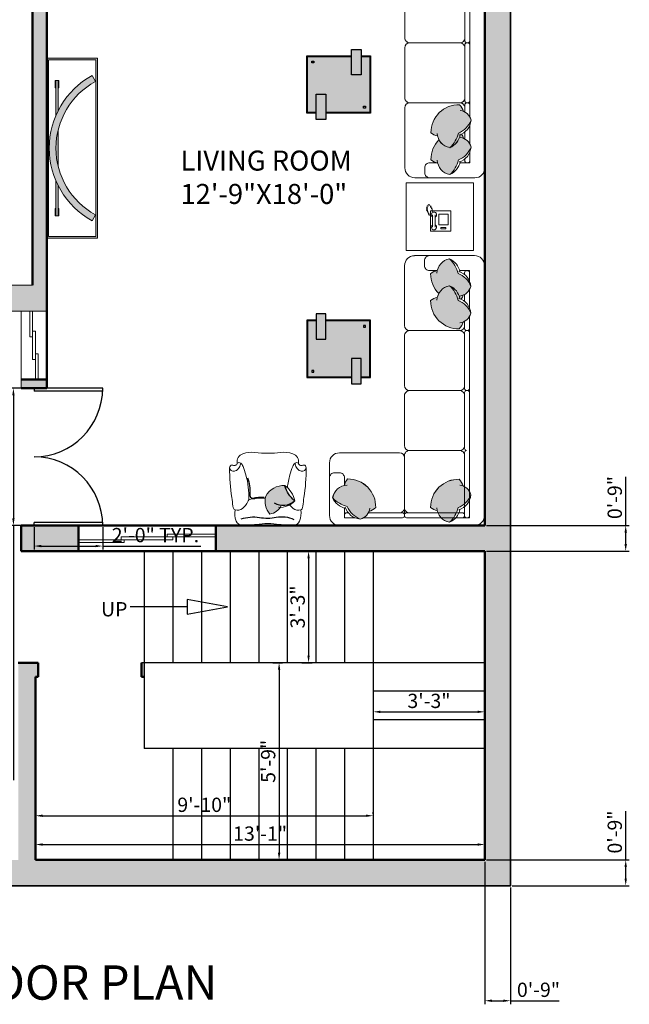
# Model space of a CAD drawing. Units: inches. Extents: x 1734 to 4011, y 1071 to 1891.
# Tile 2 of 27: x 1947 to 2160, y 1083 to 1427. Entities that reach past the tile are written whole.
import ezdxf

# ---------------------------------------------------------------- set-up
doc = ezdxf.new("R2010")
doc.units = ezdxf.units.IN
for name, color, linetype, lineweight in [('A-ANNO-DIMS', 2, 'Continuous', 18), ('A-ANNO-TEXT', 7, 'Continuous', 25), ('A-AREA-IDEN', 3, 'Continuous', 18), ('A-DOOR', 3, 'Continuous', 25), ('A-FLOR-STRS', 2, 'Continuous', 25), ('A-FURN', 8, 'Continuous', 18), ('A-FURN-PATT', 252, 'Continuous', 13), ('A-GLAZ', 4, 'Continuous', 18), ('A-WALL', 7, 'Continuous', 50), ('A-WALL-PATT', 8, 'Continuous', 13), ('aparador', 36, 'Continuous', 9), ('C-PROP', 1, 'Continuous', 35), ('moveis', 254, 'Continuous', 5)]:
    doc.layers.add(name, color=color, linetype=linetype, lineweight=lineweight)
doc.layers.add('IFF-FURN-DETAIL', color=250, linetype='Continuous')
doc.layers.add('MOBIL', color=7, linetype='Continuous')
doc.styles.get("Standard").update_dxf_attribs({"font": 'arial.ttf'})
doc.dimstyles.new('ISO-25', dxfattribs={"dimtxt": 5, "dimasz": 2.5, "dimexe": 1.25, "dimexo": 0.625, "dimtad": 1, "dimdec": 1, "dimlunit": 3, "dimtxsty": 'Standard', "dimcen": 2.5, "dimclrt": 1, "dimadec": 0, "dimazin": 0, "dimtfac": 1, "dimtdec": 1, "dimtmove": 0, "dimatfit": 3, "dimfxl": 1, "dimarcsym": 0})

# ---------------------------------------------------------------- blocks, each defined once
blk = doc.blocks.new('*D8')
at = {"layer": 'A-ANNO-DIMS', "color": 0, "lineweight": -2, "transparency": 16777216}
for p, q in [((2045.72, 1241.06), (2049.34, 1241.06)), ((2048.09, 1238.56), (2048.09, 1204.56)), ((2045.72, 1202.06), (2049.34, 1202.06))]:
    blk.add_line(p, q, dxfattribs=at)
at = {"layer": 'A-ANNO-DIMS', "color": 0, "transparency": 16777216}
for points in [[(2047.67, 1238.56), (2048.5, 1238.56), (2048.09, 1241.06)], [(2047.67, 1204.56), (2048.5, 1204.56), (2048.09, 1202.06)]]:
    blk.add_solid(points, dxfattribs=at)
at = {"layer": 'Defpoints', "color": 0, "transparency": 16777216}
for p in [(2045.09, 1241.06), (2045.09, 1202.06), (2048.09, 1202.06)]:
    blk.add_point(p, dxfattribs=at)
at = {"layer": 'A-ANNO-DIMS', "color": 0, "transparency": 16777216, "insert": (2044.91, 1221.56), "char_height": 5, "attachment_point": 5, "rotation": 90}
blk.add_mtext('3\'-3"', dxfattribs=at)
blk = doc.blocks.new('*D9')
at = {"layer": 'A-ANNO-DIMS', "color": 0, "lineweight": -2, "transparency": 16777216}
for p, q in [((2035.64, 1202.06), (2039.03, 1202.06)), ((2037.78, 1199.56), (2037.78, 1135.56)), ((2035.64, 1133.06), (2039.03, 1133.06))]:
    blk.add_line(p, q, dxfattribs=at)
at = {"layer": 'A-ANNO-DIMS', "color": 0, "transparency": 16777216}
for points in [[(2037.37, 1199.56), (2038.2, 1199.56), (2037.78, 1202.06)], [(2037.37, 1135.56), (2038.2, 1135.56), (2037.78, 1133.06)]]:
    blk.add_solid(points, dxfattribs=at)
at = {"layer": 'Defpoints', "color": 0, "transparency": 16777216}
for p in [(2035.02, 1202.06), (2035.02, 1133.06), (2037.78, 1133.06)]:
    blk.add_point(p, dxfattribs=at)
at = {"layer": 'A-ANNO-DIMS', "color": 0, "transparency": 16777216, "insert": (2034.61, 1167.56), "char_height": 5, "attachment_point": 5, "rotation": 90}
blk.add_mtext('5\'-9"', dxfattribs=at)
blk = doc.blocks.new('*D10')
at = {"layer": 'A-ANNO-DIMS', "color": 0, "lineweight": -2, "transparency": 16777216}
for p, q in [((1952.65, 1149.15), (1952.65, 1149.77)), ((1955.15, 1148.52), (2068.15, 1148.52)), ((2070.65, 1149.15), (2070.65, 1149.77))]:
    blk.add_line(p, q, dxfattribs=at)
at = {"layer": 'A-ANNO-DIMS', "color": 0, "transparency": 16777216}
for points in [[(1955.15, 1148.94), (1955.15, 1148.11), (1952.65, 1148.52)], [(2068.15, 1148.94), (2068.15, 1148.11), (2070.65, 1148.52)]]:
    blk.add_solid(points, dxfattribs=at)
at = {"layer": 'Defpoints', "color": 0, "transparency": 16777216}
for p in [(1952.65, 1148.52), (2070.65, 1148.52), (2070.65, 1148.52)]:
    blk.add_point(p, dxfattribs=at)
at = {"layer": 'A-ANNO-DIMS', "color": 0, "transparency": 16777216, "insert": (2011.65, 1151.7), "char_height": 5, "attachment_point": 5}
blk.add_mtext('9\'-10"', dxfattribs=at)
blk = doc.blocks.new('*D12')
at = {"layer": 'A-ANNO-DIMS', "color": 0, "lineweight": -2, "transparency": 16777216}
for p, q in [((1952.65, 1133.69), (1952.65, 1139.7)), ((1955.15, 1138.45), (2107.15, 1138.45)), ((2109.65, 1133.69), (2109.65, 1139.7))]:
    blk.add_line(p, q, dxfattribs=at)
at = {"layer": 'A-ANNO-DIMS', "color": 0, "transparency": 16777216}
for points in [[(1955.15, 1138.87), (1955.15, 1138.04), (1952.65, 1138.45)], [(2107.15, 1138.87), (2107.15, 1138.04), (2109.65, 1138.45)]]:
    blk.add_solid(points, dxfattribs=at)
at = {"layer": 'Defpoints', "color": 0, "transparency": 16777216}
for p in [(2109.65, 1138.45), (1952.65, 1133.06), (2109.65, 1133.06)]:
    blk.add_point(p, dxfattribs=at)
at = {"layer": 'A-ANNO-DIMS', "color": 0, "transparency": 16777216, "insert": (2031.15, 1141.63), "char_height": 5, "attachment_point": 5}
blk.add_mtext('13\'-1"', dxfattribs=at)
blk = doc.blocks.new('*D13')
at = {"layer": 'A-ANNO-DIMS', "color": 0, "lineweight": -2, "transparency": 16777216}
for p, q in [((2070.65, 1186.44), (2070.65, 1183.62)), ((2073.15, 1184.87), (2107.15, 1184.87)), ((2109.65, 1185.49), (2109.65, 1186.12))]:
    blk.add_line(p, q, dxfattribs=at)
at = {"layer": 'A-ANNO-DIMS', "color": 0, "transparency": 16777216}
for points in [[(2073.15, 1185.28), (2073.15, 1184.45), (2070.65, 1184.87)], [(2107.15, 1185.28), (2107.15, 1184.45), (2109.65, 1184.87)]]:
    blk.add_solid(points, dxfattribs=at)
at = {"layer": 'Defpoints', "color": 0, "transparency": 16777216}
for p in [(2070.65, 1187.06), (2109.65, 1184.87), (2109.65, 1184.87)]:
    blk.add_point(p, dxfattribs=at)
at = {"layer": 'A-ANNO-DIMS', "color": 0, "transparency": 16777216, "insert": (2090.15, 1188.05), "char_height": 5, "attachment_point": 5}
blk.add_mtext('3\'-3"', dxfattribs=at)
blk = doc.blocks.new("MD D 4'")
for p, q in [((0, 24), (0, 0)), ((1, 24), (1, 0)), ((47, 24), (47, 0)), ((48, 24), (48, 0)), ((0, 0), (1, 0)), ((48, 0), (47, 0))]:
    blk.add_line(p, q)
for centre, start, end in [((0, 0), 0, 90), ((48, 0), 90, 180)]:
    blk.add_arc(centre, 24, start, end)
blk = doc.blocks.new('Aparador ORGANICA Formatto')
at = {"layer": 'aparador', "ltscale": 0.3}
h = blk.add_hatch(color=256, dxfattribs=at)
h.dxf.hatch_style = 1
h.set_gradient(color1=(118, 213, 123), color2=(52, 168, 57), one_color=1, tint=0.43, name='INVCURVED')
h.paths.add_polyline_path([(0.8, 0.45), (-0.8, 0.45), (-0.8, 0), (0.8, 0)])
h.paths.add_polyline_path([(0.785, 0.435), (0.785, 0.015), (-0.785, 0.015), (-0.785, 0.435)], flags=16)
h.paths.add_polyline_path([(0.2911, 0.3699), (0.5365, 0.3699), (0.5365, 0.3757), (0.6011, 0.3757), (0.6011, 0.3699), (0.6011, 0.3499), (0.6011, 0.3441), (0.5365, 0.3441), (0.5365, 0.3499), (0.3338, 0.3499, -0.150336), (0.6449, 0.0488), (0.5923, 0.0199, 0.208852), (0.1632, 0.3499), (-0.1632, 0.3499, 0.208852), (-0.5923, 0.0199), (-0.6449, 0.0488, -0.150336), (-0.3338, 0.3499), (-0.5365, 0.3499), (-0.5365, 0.3441), (-0.6011, 0.3441), (-0.6011, 0.3499), (-0.6011, 0.3699), (-0.6011, 0.3757), (-0.5365, 0.3757), (-0.5365, 0.3699), (-0.2911, 0.3699, -0.206106)], flags=0)
h = blk.add_hatch(color=256, dxfattribs=at)
h.dxf.hatch_style = 1
h.set_gradient(color1=(135, 92, 69), color2=(0, 0, 0), one_color=1, name='INVCURVED')
h.paths.add_polyline_path([(-0.6449, 0.0488), (-0.5923, 0.0199, -0.590888), (0.5923, 0.0199), (0.6449, 0.0488, 0.590888)])
h = blk.add_hatch(color=256, dxfattribs=at)
h.dxf.hatch_style = 1
h.set_gradient(color1=(178, 189, 189), one_color=1, tint=1, name='CYLINDER')
h.paths.add_polyline_path([(-0.5365, 0.3757), (-0.6011, 0.3757), (-0.6011, 0.3699), (-0.5365, 0.3699)])
h.paths.add_polyline_path([(-0.5365, 0.3499), (-0.6011, 0.3499), (-0.6011, 0.3441), (-0.5365, 0.3441)])
h = blk.add_hatch(color=256, dxfattribs=at)
h.dxf.hatch_style = 1
h.set_gradient(color1=(118, 213, 123), color2=(31, 101, 35), one_color=1, tint=0.26, name='INVCURVED')
h.paths.add_polyline_path([(-0.2911, 0.3699), (-0.6011, 0.3699), (-0.6011, 0.3499), (-0.3338, 0.3499, -0.015999)])
h = blk.add_hatch(color=256, dxfattribs=at)
h.dxf.hatch_style = 1
h.set_gradient(color1=(118, 213, 123), color2=(31, 101, 35), one_color=1, tint=0.26, name='INVCURVED')
h.paths.add_polyline_path([(-0.1632, 0.3499), (0.1632, 0.3499, 0.122516)])
h = blk.add_hatch(color=256, dxfattribs=at)
h.dxf.hatch_style = 1
h.set_gradient(color1=(118, 213, 123), color2=(31, 101, 35), one_color=1, tint=0.26, name='INVCURVED')
h.paths.add_polyline_path([(0.6011, 0.3699), (0.2911, 0.3699, -0.015999), (0.3338, 0.3499), (0.6011, 0.3499)])
h = blk.add_hatch(color=256, dxfattribs=at)
h.dxf.hatch_style = 1
h.set_gradient(color1=(178, 189, 189), one_color=1, tint=1, name='CYLINDER')
h.paths.add_polyline_path([(0.6011, 0.3757), (0.5365, 0.3757), (0.5365, 0.3699), (0.6011, 0.3699)])
h.paths.add_polyline_path([(0.6011, 0.3499), (0.5365, 0.3499), (0.5365, 0.3441), (0.6011, 0.3441)])
for p, q in [((-0.5923, 0.0199), (-0.6449, 0.0488)), ((0.5923, 0.0199), (0.6449, 0.0488))]:
    blk.add_line(p, q, dxfattribs=at)
for points in [[(-0.6011, 0.3699), (-0.6011, 0.3757), (-0.5365, 0.3757), (-0.5365, 0.3699)], [(0.6011, 0.3699), (0.6011, 0.3757), (0.5365, 0.3757), (0.5365, 0.3699)], [(-0.5365, 0.3499), (-0.5365, 0.3441), (-0.6011, 0.3441), (-0.6011, 0.3499)], [(0.5365, 0.3499), (0.5365, 0.3441), (0.6011, 0.3441), (0.6011, 0.3499)]]:
    blk.add_lwpolyline(points, dxfattribs=at)
for radius in [0.7362, 0.6762]:
    blk.add_arc((0, -0.3063), radius, 28.84335, 151.15665, dxfattribs=at)
at = {"layer": 'moveis', "ltscale": 0.3}
for p, q in [((-0.6011, 0.3699), (-0.6011, 0.3499)), ((-0.2911, 0.3699), (-0.6011, 0.3699)), ((0.2911, 0.3699), (0.6011, 0.3699)), ((0.6011, 0.3699), (0.6011, 0.3499)), ((-0.6011, 0.3499), (-0.3338, 0.3499)), ((-0.1632, 0.3499), (0.1632, 0.3499)), ((0.6011, 0.3499), (0.3338, 0.3499))]:
    blk.add_line(p, q, dxfattribs=at)
for points in [[(-0.8, 0), (0.8, 0), (0.8, 0.45), (-0.8, 0.45)], [(-0.785, 0.015), (0.785, 0.015), (0.785, 0.435), (-0.785, 0.435)]]:
    blk.add_lwpolyline(points, close=True, dxfattribs=at)
blk = doc.blocks.new('Mesa de centro Cantria feeling')
at = {"layer": 'MOBIL', "ltscale": 0.2}
h = blk.add_hatch(color=256, dxfattribs=at)
h.set_gradient(color1=(74, 55, 38), color2=(104, 77, 54), one_color=1, tint=0.31, name='CYLINDER')
h.paths.add_polyline_path([(-0.85, -0.3), (-0.7, -0.3), (-0.7, 0.1), (-0.85, 0.1)])
h = blk.add_hatch(color=256, dxfattribs=at)
h.set_gradient(color1=(221, 221, 223), one_color=1, tint=1)
h.paths.add_polyline_path([(-0.15, -0.6), (-0.15, -0.89), (-0.01, -0.89), (-0.01, -0.01), (-0.7, -0.01), (-0.7, -0.3), (-0.85, -0.3), (-0.85, -0.01), (-0.99, -0.01), (-0.99, -0.89), (-0.3, -0.89), (-0.3, -0.6)])
h.paths.add_polyline_path([(-0.112, -0.112), (-0.112, -0.082), (-0.082, -0.082), (-0.082, -0.112)], flags=16)
h.paths.add_polyline_path([(-0.888, -0.788), (-0.888, -0.818), (-0.918, -0.818), (-0.918, -0.788)], flags=16)
h = blk.add_hatch(color=256, dxfattribs=at)
h.set_gradient(color1=(74, 55, 38), color2=(104, 77, 54), one_color=1, tint=0.31, name='CYLINDER')
h.paths.add_polyline_path([(-0.15, -0.6), (-0.3, -0.6), (-0.3, -1), (-0.15, -1)])
for points in [[(-0.85, 0), (-1, 0), (-1, -0.9), (-0.3, -0.9)], [(-0.15, -0.9), (0, -0.9), (0, 0), (-0.7, 0)], [(-0.85, -0.01), (-0.99, -0.01), (-0.99, -0.89), (-0.3, -0.89)], [(-0.15, -0.89), (-0.01, -0.89), (-0.01, -0.01), (-0.7, -0.01)]]:
    blk.add_lwpolyline(points, dxfattribs=at)
for points in [[(-0.85, -0.3), (-0.7, -0.3), (-0.7, 0.1), (-0.85, 0.1)], [(-0.082, -0.082), (-0.112, -0.082), (-0.112, -0.112), (-0.082, -0.112)], [(-0.15, -0.6), (-0.3, -0.6), (-0.3, -1), (-0.15, -1)], [(-0.918, -0.818), (-0.888, -0.818), (-0.888, -0.788), (-0.918, -0.788)]]:
    blk.add_lwpolyline(points, close=True, dxfattribs=at)
blk = doc.blocks.new('SOFA 1')
at = {"transparency": 33554687}
h = blk.add_hatch(color=256, dxfattribs=at)
h.dxf.hatch_style = 1
h.paths.add_polyline_path([(3723.52, 1308.63, 0.147724), (3717.76, 1305.24, 0.310469), (3722.42, 1300.4), (3722.42, 1300.25, 0.156703), (3723.62, 1297.8, 0.425821), (3734.69, 1309.08, 0.121928), (3732.05, 1310.63, 0.233216), (3728.6, 1313.59, 0.213835)])
h = blk.add_hatch(color=256, dxfattribs=at)
h.dxf.hatch_style = 1
h.paths.add_polyline_path([(3769.65, 1307.6, 0.084911), (3767.15, 1309.12, 0.046133), (3766.46, 1311.13), (3759.18, 1311.13, 0.039409), (3758.92, 1310.24, 0.165523), (3756.31, 1309.02, 0.42585), (3767.59, 1297.95, 0.121928), (3769.15, 1300.58, 0.027403), (3769.65, 1300.83)])
h.paths.add_polyline_path([(3765.34, 1313.08), (3760.4, 1313.08, 0.097704), (3759.18, 1311.13), (3766.46, 1311.13, 0.04873)])
h.paths.add_polyline_path([(3763.76, 1314.88, 0.16488), (3760.4, 1313.08), (3765.34, 1313.08, 0.051917)])
h.paths.add_polyline_path([(3771.6, 1305.17, 0.090388), (3769.65, 1307.6), (3769.65, 1300.83, 0.136035), (3771.6, 1302.77)])
h = blk.add_hatch(color=256, dxfattribs=at)
h.dxf.hatch_style = 1
h.paths.add_polyline_path([(3769.16, 1235.96, 0.122267), (3767.6, 1238.61, 0.425972), (3756.32, 1227.54, 0.165563), (3758.93, 1226.32, 0.309481), (3763.76, 1221.69, 0.002677), (3763.83, 1221.72, 0.146094), (3767.16, 1227.43, 0.212433), (3772.1, 1232.48, 0.235342)])
h = blk.add_hatch(color=256, dxfattribs=at)
h.dxf.hatch_style = 1
h.paths.add_polyline_path([(3769.16, 1225.36, 0.122267), (3767.6, 1228.01, 0.425972), (3756.32, 1216.94, 0.165563), (3758.93, 1215.72, 0.309481), (3763.76, 1211.09, 0.002677), (3763.83, 1211.12, 0.146094), (3767.16, 1216.83, 0.212433), (3772.1, 1221.88, 0.235342)])
for p, q in [((3720.45, 1316.13), (3773.58, 1316.13)), ((3777.51, 1312.19), (3777.51, 1213.72))]:
    blk.add_line(p, q, dxfattribs=at)
for points in [[(3716.51, 1312.2), (3716.51, 1291.44)], [(3722.42, 1313.08), (3722.42, 1309.23), (3722.42, 1313.08), (3726.57, 1313.08)], [(3729.85, 1313.08), (3745.25, 1313.08)], [(3746.01, 1312.3), (3746.01, 1288.55)], [(3768.11, 1313.08), (3746.78, 1313.08)], [(3771.6, 1313.08), (3767.75, 1313.08), (3771.6, 1313.08), (3771.6, 1308.93)], [(3769.66, 1287.39), (3769.65, 1312.3)], [(3771.6, 1313.08), (3771.61, 1233.74)], [(3723.21, 1311.13), (3723.93, 1311.13)], [(3731.82, 1311.13), (3745.25, 1311.13)], [(3746.01, 1310.97), (3746.01, 1311.36)], [(3746.01, 1288.54), (3746.01, 1308.23)], [(3768.87, 1311.13), (3746.78, 1311.13)], [(3769.65, 1309.43), (3769.65, 1308.71)], [(3722.42, 1300.39), (3722.42, 1297.33)], [(3720.45, 1295.38), (3718.48, 1295.38)], [(3720.45, 1287.5), (3744.09, 1287.5)], [(3746.02, 1284.63), (3746.02, 1264.94)], [(3747.99, 1286.6), (3767.69, 1286.6)], [(3769.66, 1263.75), (3769.66, 1285.81)], [(3769.66, 1277.18), (3769.66, 1263.75)], [(3747.99, 1262.97), (3767.69, 1262.97)], [(3769.66, 1240.12), (3769.66, 1262.18)], [(3770.43, 1262.97), (3770.82, 1262.97)], [(3746.02, 1260.99), (3746.02, 1241.3)], [(3747.99, 1239.33), (3767.69, 1239.33)], [(3769.66, 1235.71), (3769.66, 1238.54)], [(3770.43, 1239.33), (3770.82, 1239.33)], [(3746.02, 1237.36), (3746.02, 1213.74)], [(3771.61, 1223.14), (3771.61, 1230.47)], [(3769.66, 1225.11), (3769.66, 1227.82)], [(3767.76, 1215.72), (3771.61, 1215.72), (3771.61, 1219.84), (3771.61, 1215.72)], [(3755.86, 1215.72), (3758.92, 1215.72)], [(3769.66, 1216.5), (3769.66, 1217.22)], [(3753.91, 1211.77), (3753.91, 1213.74)], [(3749.97, 1209.8), (3773.58, 1209.8)]]:
    blk.add_lwpolyline(points, close=True, dxfattribs=at)
for points in [[(3717.76, 1305.24, -0.147724), (3723.52, 1308.63, -0.213355), (3728.59, 1313.59, 0.213355), (3723.52, 1308.63, 0.147724), (3717.76, 1305.24, -0.249545), (3722.86, 1309.34, 0.249545), (3717.75, 1305.25, 0.356779), (3723.4, 1300.28, -0.356779), (3717.76, 1305.24)], [(3728.58, 1313.6, -0.306333), (3732.42, 1309.31, 0.306333), (3728.58, 1313.6, 0.306674), (3722.72, 1308.89, -0.306674), (3728.58, 1313.6)], [(3763.76, 1314.88, -0.147724), (3767.15, 1309.12, -0.213355), (3772.1, 1304.05, 0.213355), (3767.15, 1309.12, 0.147724), (3763.76, 1314.88, -0.249545), (3767.86, 1309.77, 0.249545), (3763.77, 1314.89, 0.356779), (3758.8, 1309.23, -0.356779), (3763.76, 1314.88)], [(3734.69, 1309.08, -0.425972), (3723.62, 1297.8, -0.165552), (3722.4, 1300.4, 0.165552), (3723.62, 1297.79, 0.425972), (3734.69, 1309.07, 0.121514), (3732.07, 1310.63, -0.121514), (3734.69, 1309.08)], [(3767.6, 1297.95, -0.425972), (3756.31, 1309.01, -0.165552), (3758.92, 1310.24, 0.165552), (3756.31, 1309.02, 0.425972), (3767.59, 1297.95, 0.121514), (3769.14, 1300.57, -0.121514), (3767.6, 1297.95)], [(3772.11, 1304.06, -0.306333), (3767.83, 1300.22, 0.306333), (3772.11, 1304.06, 0.306674), (3767.4, 1309.91, -0.306674), (3772.11, 1304.06)], [(3770.44, 1286.63, -0.414214), (3769.66, 1287.4, 0.414214), (3770.44, 1286.63, 0.414214), (3769.66, 1285.83, -0.414214), (3770.44, 1286.63)], [(3748.01, 1262.99, -0.414214), (3746.05, 1264.95, 0.414214), (3748.01, 1262.97, 0.414213), (3746.05, 1261.01, -0.414213), (3748.01, 1262.99)], [(3770.44, 1262.99, -0.414214), (3769.66, 1263.77, 0.414214), (3770.44, 1262.99, 0.414214), (3769.66, 1262.19, -0.414214), (3770.44, 1262.99)], [(3770.83, 1262.97, -0.414214), (3771.61, 1262.19, 0.414214), (3770.83, 1262.99, 0.414214), (3771.61, 1263.77, -0.414214), (3770.83, 1262.97)], [(3748.01, 1239.35, -0.414214), (3746.05, 1241.31, 0.414214), (3748.01, 1239.33, 0.414213), (3746.05, 1237.37, -0.414213), (3748.01, 1239.35)], [(3756.32, 1227.54, -0.425972), (3767.6, 1238.61, -0.121514), (3769.16, 1235.98, 0.121514), (3767.6, 1238.61, 0.425972), (3756.32, 1227.54, 0.165552), (3758.93, 1226.32, -0.165552), (3756.32, 1227.54)], [(3767.7, 1239.33, -0.414214), (3769.66, 1237.37, 0.414214), (3767.7, 1239.35, 0.414214), (3769.66, 1241.31, -0.414214), (3767.7, 1239.33)], [(3770.44, 1239.35, -0.414214), (3769.66, 1240.13, 0.414214), (3770.44, 1239.33, 0.414214), (3769.66, 1238.55, -0.414214), (3770.44, 1239.35)], [(3770.83, 1239.33, -0.414214), (3771.61, 1238.55, 0.414214), (3770.83, 1239.35, 0.414214), (3771.61, 1240.13, -0.414214), (3770.83, 1239.33)], [(3772.1, 1232.5, -0.306674), (3767.41, 1226.64, 0.306674), (3772.1, 1232.5, 0.306333), (3767.84, 1236.34, -0.306333), (3772.1, 1232.5)], [(3763.78, 1221.67, 0.249545), (3767.87, 1226.78, -0.249545), (3763.76, 1221.69, -0.356779), (3758.81, 1227.32, 0.356779), (3763.77, 1221.68, 0.147724), (3767.16, 1227.43, 0.213355), (3772.11, 1232.51, -0.213355), (3767.16, 1227.43, -0.147724), (3763.78, 1221.67)], [(3756.32, 1216.94, -0.200233), (3759.49, 1224.76, 0.200233), (3756.32, 1216.94, 0.165552), (3758.93, 1215.72, -0.165552), (3756.32, 1216.94)], [(3772.1, 1221.9, -0.306674), (3767.41, 1216.04, 0.306674), (3772.1, 1221.9, -0.213355), (3767.16, 1216.83, -0.147724), (3763.77, 1211.08, 0.147724), (3767.15, 1216.83, 0.213355), (3772.1, 1221.9)], [(3763.76, 1211.09, -0.356779), (3758.81, 1216.72, 0.356779), (3763.76, 1211.09, 0.249545), (3767.87, 1216.18, -0.249545), (3763.76, 1211.09)]]:
    blk.add_lwpolyline(points, format="xyb", dxfattribs=at)
for points in [[(3722.42, 1311.91, 0.414214), (3723.2, 1311.13, -0.414214)], [(3770.43, 1313.08, 0.414214), (3769.65, 1312.3, -0.414214)], [(3771.6, 1312.3, 0.414214), (3770.82, 1313.08, -0.414214)], [(3716.51, 1297.34, 0.414214), (3718.47, 1295.38, -0.414214)], [(3720.44, 1295.38, 0.414214), (3722.4, 1297.34, -0.414214)], [(3716.51, 1291.45, 0.414212), (3720.44, 1287.52, -0.414212)], [(3746.03, 1288.56, 0.414214), (3747.99, 1286.6, 0.414213), (3746.03, 1284.64, -0.414213), (3747.99, 1286.6, -0.414214)], [(3769.66, 1284.64, 0.414214), (3767.7, 1286.6, 0.414214), (3769.66, 1288.56, -0.414214), (3767.7, 1286.6, -0.414214)], [(3769.66, 1261.01, 0.414214), (3767.7, 1262.97, 0.414214), (3769.66, 1264.93, -0.414214), (3767.7, 1262.97, -0.414214)], [(3769.16, 1225.36, 0.071861), (3768.39, 1227.01, -0.071861)], [(3772.13, 1221.9, 0.306333), (3767.84, 1225.74, -0.306333)], [(3755.87, 1215.72, 0.414214), (3753.91, 1213.76, -0.414214)], [(3769.66, 1216.52, 0.414214), (3770.44, 1215.74, -0.414214)], [(3770.83, 1215.74, 0.414214), (3771.61, 1216.52, -0.414214)], [(3746.05, 1213.76, 0.414212), (3749.98, 1209.82, -0.414212)], [(3755.87, 1209.8, -0.414214), (3753.91, 1211.76, 0.414214)]]:
    blk.add_lwpolyline(points, format="xyb", close=True, dxfattribs=at)
for centre, radius, start, end in [((3720.44, 1312.2), 3.93, 90.0002, 179.9998), ((3720.44, 1312.19), 3.94, 89.9158, 179.9154), ((3773.58, 1312.2), 3.93, 0.0002, 89.9998), ((3773.57, 1312.19), 3.94, 359.9158, 89.9154), ((3745.22, 1312.29), 0.789, 0.8425, 90.8425), ((3745.24, 1311.91), 0.777, 270, 0), ((3745.24, 1311.91), 0.777, 270, 0), ((3746.8, 1312.29), 0.789, 89.1575, 179.1575), ((3746.79, 1311.91), 0.777, 180, 270), ((3746.79, 1311.91), 0.777, 180, 270), ((3768.87, 1312.3), 0.777, 360, 90), ((3768.87, 1311.91), 0.777, 270, 0), ((3744.09, 1309.21), 1.92, 358.766, 90.5111), ((3747.93, 1309.21), 1.92, 89.4889, 181.234), ((3744.08, 1289.48), 1.96, 270, 360), ((3744.08, 1289.48), 1.96, 270, 360), ((3773.58, 1213.73), 3.93, 270.0002, 359.9998), ((3773.59, 1213.73), 3.93, 269.9156, 359.9152)]:
    blk.add_arc(centre, radius, start, end, dxfattribs=at)
blk = doc.blocks.new('PILLOW-1')
at = {"color": 0}
blk.add_lwpolyline([(198, -165, -0.232884), (126, -346, -0.184752), (-44, -234, -0.286563), (75, -22, -0.237978), (273, -68, -0.243587), (179, -195, 4.263709)], format="xyb", dxfattribs=at)
at = {"layer": 'IFF-FURN-DETAIL'}
blk.add_lwpolyline([(148, -118, -0.343333), (126, -342, 0.126408), (-40, -233, -5.969376)], format="xyb", dxfattribs=at)
blk = doc.blocks.new('CLNG90')
for points in [[(689, 370, 0.157831), (677, 385, 0.121013), (646, 395, -0.017334), (547, 407, 0.041496), (215, 431, 0.153531), (191, 423, 0.382906), (185, 395, -0.284047), (184, 361, 0.011997), (177, 351, -0.370479), (160, 345, 0.380647), (56, 282, 0.117468), (41, 146, -0.027775), (50, 0, -8.773898)], [(160, 345, 0.22481), (160, 306, 0.055398), (209, 322, 0.180116), (249, 368, 0.194833), (248, 405, 0.242377), (215, 431, 1.52074)], [(160, 345, 0.22481), (160, 306, 0.055398), (209, 322, 0.180116), (249, 368, 0.194833), (248, 405, 0.242377), (215, 431, 1.52074)], [(689, 370, -0.235486), (671, 286, -0.134038), (574, 215, -0.079303), (293, 248, -0.027048), (199, 280, -0.106276), (160, 306, -1.699)], [(689, 370, -0.235486), (671, 286, -0.134038), (574, 215, -0.079303), (293, 248, -0.027048), (199, 280, -0.106276), (160, 306, -1.699)], [(689, 370, -0.146607), (814, 357, -0.305296), (862, 286, -0.042137), (852, 131, 0.040285), (843, 0, 3.952121)], [(574, 215, 0.061244), (556, 29, 3.376255)], [(574, 215, 0.061244), (556, 29, 3.376255)], [(689, -370, -0.157831), (677, -385, -0.121013), (646, -395, 0.017334), (547, -407, -0.041496), (215, -431, -0.153531), (191, -423, -0.382906), (185, -395, 0.284047), (184, -361, -0.011997), (177, -351, 0.370479), (160, -345, -0.380647), (56, -282, -0.117468), (41, -146, 0.027775), (50, 0, 8.773898)], [(689, -370, 0.146607), (814, -357, 0.305296), (862, -286, 0.042137), (852, -131, -0.040285), (843, 0, -3.952121)], [(437, -220, 0.041086), (293, -248, 0.027048), (199, -280, 0.106276), (160, -306, 1.699)], [(437, -220, 0.041086), (293, -248, 0.027048), (199, -280, 0.106276), (160, -306, 1.699)], [(160, -345, -0.22481), (160, -306, -0.055398), (209, -322, -0.180116), (249, -368, -0.194833), (248, -405, -0.242377), (215, -431, -1.52074)], [(160, -345, -0.22481), (160, -306, -0.055398), (209, -322, -0.180116), (249, -368, -0.194833), (248, -405, -0.242377), (215, -431, -1.52074)], [(689, -370, 0.235486), (671, -286, 0.060693), (632, -247, 0.001296)], [(689, -370, 0.235486), (671, -286, 0.060693), (632, -247, 0.001296)]]:
    blk.add_lwpolyline(points, format="xyb")
at = {"layer": 'IFF-FURN-DETAIL'}
for points in [[(328, 228, 0.109125), (508, 203, -0.16587), (546, 194, -0.314359), (555, 172, 0.072017), (544, 42, 4.351186)], [(328, 228, 0.109125), (508, 203, -0.16587), (546, 194, -0.314359), (555, 172, 0.072017), (544, 42, 4.351186)], [(791, 301, 0.124986), (774, 96, -0.091334), (771, -95, 0.164688), (797, -292, 1.068868)], [(791, 301, 0.124986), (774, 96, -0.091334), (771, -95, 0.164688), (797, -292, 1.068868)]]:
    blk.add_lwpolyline(points, format="xyb", dxfattribs=at)
at = {"xscale": 1.016, "yscale": 1.016, "zscale": 1.016}
blk.add_blockref('PILLOW-1', (458, 47), dxfattribs=at)
blk.add_blockref('PILLOW-1', (458, 47), dxfattribs=at)
blk = doc.blocks.new('*D75')
at = {"layer": 'A-ANNO-DIMS', "color": 0, "lineweight": -2, "transparency": 16777216}
for p, q in [((1951.52, 1298.06), (1943.7, 1298.06)), ((1944.95, 1295.56), (1944.95, 1252.56)), ((1951.52, 1250.06), (1943.7, 1250.06)), ((1944.95, 1250.06), (1944.95, 1160.96))]:
    blk.add_line(p, q, dxfattribs=at)
at = {"layer": 'A-ANNO-DIMS', "color": 0, "transparency": 16777216}
for points in [[(1944.53, 1295.56), (1945.37, 1295.56), (1944.95, 1298.06)], [(1944.53, 1252.56), (1945.37, 1252.56), (1944.95, 1250.06)]]:
    blk.add_solid(points, dxfattribs=at)
at = {"layer": 'Defpoints', "color": 0, "transparency": 16777216}
for p in [(1952.15, 1298.06), (1944.95, 1250.06), (1952.15, 1250.06)]:
    blk.add_point(p, dxfattribs=at)
at = {"layer": 'A-ANNO-DIMS', "color": 1, "transparency": 16777216, "insert": (1941.74, 1204.26), "char_height": 5, "attachment_point": 5, "rotation": 90}
blk.add_mtext('MAIN DOOR MD 4\'-0" TYP.', dxfattribs=at)
blk = doc.blocks.new('*D76')
at = {"layer": 'A-ANNO-DIMS', "color": 0, "lineweight": -2, "transparency": 16777216}
for p, q in [((1952.15, 1249.44), (1952.15, 1241.61)), ((1976.15, 1249.44), (1976.15, 1241.61)), ((1954.65, 1242.86), (1973.65, 1242.86)), ((1976.15, 1242.86), (2010.46, 1242.86))]:
    blk.add_line(p, q, dxfattribs=at)
at = {"layer": 'A-ANNO-DIMS', "color": 0, "transparency": 16777216}
for points in [[(1954.65, 1243.28), (1954.65, 1242.44), (1952.15, 1242.86)], [(1973.65, 1243.28), (1973.65, 1242.44), (1976.15, 1242.86)]]:
    blk.add_solid(points, dxfattribs=at)
at = {"layer": 'Defpoints', "color": 0, "transparency": 16777216}
for p in [(1952.15, 1250.06), (1976.15, 1250.06), (1976.15, 1242.86)]:
    blk.add_point(p, dxfattribs=at)
at = {"layer": 'A-ANNO-DIMS', "color": 1, "transparency": 16777216, "insert": (1994.56, 1246.04), "char_height": 5, "attachment_point": 5}
blk.add_mtext('2\'-0" TYP.', dxfattribs=at)
blk = doc.blocks.new('*D108')
at = {"layer": 'A-ANNO-DIMS', "color": 0, "lineweight": -2, "transparency": 16777216}
for p, q in [((2158.9, 1133.06), (2158.9, 1150.1)), ((2110.27, 1133.06), (2160.15, 1133.06)), ((2158.9, 1126.56), (2158.9, 1130.56)), ((2119.27, 1124.06), (2160.15, 1124.06))]:
    blk.add_line(p, q, dxfattribs=at)
at = {"layer": 'A-ANNO-DIMS', "color": 0, "transparency": 16777216}
for points in [[(2158.48, 1130.56), (2159.32, 1130.56), (2158.9, 1133.06)], [(2158.48, 1126.56), (2159.32, 1126.56), (2158.9, 1124.06)]]:
    blk.add_solid(points, dxfattribs=at)
at = {"layer": 'Defpoints', "color": 0, "transparency": 16777216}
for p in [(2109.65, 1133.06), (2158.9, 1133.06), (2118.65, 1124.06)]:
    blk.add_point(p, dxfattribs=at)
at = {"layer": 'A-ANNO-DIMS', "color": 1, "transparency": 16777216, "insert": (2155.72, 1142.83), "char_height": 5, "attachment_point": 5, "rotation": 90}
blk.add_mtext('0\'-9"', dxfattribs=at)
blk = doc.blocks.new('*D109')
at = {"layer": 'A-ANNO-DIMS', "color": 0, "lineweight": -2, "transparency": 16777216}
for p, q in [((2158.9, 1250.06), (2158.9, 1267.1)), ((2110.27, 1250.06), (2160.15, 1250.06)), ((2158.9, 1243.56), (2158.9, 1247.56)), ((2110.27, 1241.06), (2160.15, 1241.06))]:
    blk.add_line(p, q, dxfattribs=at)
at = {"layer": 'A-ANNO-DIMS', "color": 0, "transparency": 16777216}
for points in [[(2158.48, 1247.56), (2159.32, 1247.56), (2158.9, 1250.06)], [(2158.48, 1243.56), (2159.32, 1243.56), (2158.9, 1241.06)]]:
    blk.add_solid(points, dxfattribs=at)
at = {"layer": 'Defpoints', "color": 0, "transparency": 16777216}
for p in [(2109.65, 1250.06), (2158.9, 1250.06), (2109.65, 1241.06)]:
    blk.add_point(p, dxfattribs=at)
at = {"layer": 'A-ANNO-DIMS', "color": 1, "transparency": 16777216, "insert": (2155.72, 1259.83), "char_height": 5, "attachment_point": 5, "rotation": 90}
blk.add_mtext('0\'-9"', dxfattribs=at)
blk = doc.blocks.new('*D110')
at = {"layer": 'A-ANNO-DIMS', "color": 0, "lineweight": -2, "transparency": 16777216}
for p, q in [((2109.65, 1132.44), (2109.65, 1082.56)), ((2118.65, 1123.44), (2118.65, 1082.56)), ((2112.15, 1083.81), (2116.15, 1083.81)), ((2118.65, 1083.81), (2135.69, 1083.81))]:
    blk.add_line(p, q, dxfattribs=at)
at = {"layer": 'A-ANNO-DIMS', "color": 0, "transparency": 16777216}
for points in [[(2112.15, 1084.23), (2112.15, 1083.39), (2109.65, 1083.81)], [(2116.15, 1084.23), (2116.15, 1083.39), (2118.65, 1083.81)]]:
    blk.add_solid(points, dxfattribs=at)
at = {"layer": 'Defpoints', "color": 0, "transparency": 16777216}
for p in [(2109.65, 1133.06), (2118.65, 1124.06), (2118.65, 1083.81)]:
    blk.add_point(p, dxfattribs=at)
at = {"layer": 'A-ANNO-DIMS', "color": 1, "transparency": 16777216, "insert": (2128.42, 1086.99), "char_height": 5, "attachment_point": 5}
blk.add_mtext('0\'-9"', dxfattribs=at)

msp = doc.modelspace()

# ---------------------------------------------------------------- hatches: boundary and pattern name
at = {"layer": 'A-FURN-PATT'}
h = msp.add_hatch(color=256, dxfattribs=at)
h.dxf.hatch_style = 1
h.paths.add_polyline_path([(2033.08, 1260.29, 0.237978), (2034.54, 1254.06, 0.250405), (2038.61, 1257.12, 0.218011), (2043.17, 1258.66, -0.129718), (2039.67, 1264.05, 0.283254)])
at = {"layer": 'A-WALL-PATT'}
h = msp.add_hatch(color=256, dxfattribs=at)
h.dxf.hatch_style = 1
h.paths.add_polyline_path([(1857.65, 1835.06), (1857.65, 1793.06), (1862.65, 1793.06), (1862.65, 1835.06), (1951.65, 1835.06), (1951.65, 1763.06), (1897.65, 1763.06), (1897.65, 1758.06), (1951.65, 1758.06), (1951.65, 1617.06), (1956.65, 1617.06), (1956.65, 1758.06), (2009.65, 1758.06), (2009.65, 1763.06), (1956.65, 1763.06), (1956.65, 1835.06), (2044.65, 1835.06), (2044.65, 1763.06), (2039.65, 1763.06), (2039.65, 1758.06), (2054.65, 1758.06), (2054.65, 1763.06), (2049.65, 1763.06), (2049.65, 1835.06), (2109.65, 1835.06), (2109.65, 1763.06), (2084.65, 1763.06), (2084.65, 1758.06), (2109.65, 1758.06), (2109.65, 1530.06), (2095.15, 1530.06), (2095.15, 1525.06), (2109.65, 1525.06), (2109.65, 1471.06), (2089.15, 1471.06), (2089.15, 1466.06), (2109.65, 1466.06), (2109.65, 1250.06), (2015.65, 1250.06), (2015.65, 1241.06), (2109.65, 1241.06), (2109.65, 1133.06), (1952.65, 1133.06), (1952.65, 1197.06), (1953.65, 1197.06), (1953.65, 1202.06), (1946.65, 1202.06), (1946.65, 1133.06), (1934.65, 1133.06), (1934.65, 1124.06), (2118.65, 1124.06), (2118.65, 1844.06), (1758.65, 1844.06), (1758.65, 1758.06), (1773.65, 1758.06), (1773.65, 1763.06), (1767.65, 1763.06), (1767.65, 1835.06)])
h.paths.add_polyline_path([(1803.65, 1649.06), (1812.65, 1649.06), (1812.65, 1758.06), (1867.65, 1758.06), (1867.65, 1763.06), (1797.65, 1763.06), (1797.65, 1758.06), (1803.65, 1758.06)], flags=17)
h.paths.add_polyline_path([(1803.65, 1572.06), (1956.65, 1572.06), (1956.65, 1581.06), (1951.65, 1581.06), (1951.65, 1577.06), (1812.65, 1577.06), (1812.65, 1601.06), (1803.65, 1601.06)], flags=17)
h.paths.add_polyline_path([(2044.65, 1530.06), (2044.65, 1525.06), (2059.15, 1525.06), (2059.15, 1530.06)], flags=17)
h.paths.add_polyline_path([(2009.65, 1466.06), (2035.15, 1466.06), (2035.15, 1471.06), (2014.65, 1471.06), (2014.65, 1530.06), (2009.65, 1530.06)], flags=17)
h.paths.add_polyline_path([(1896.65, 1537.06), (1896.65, 1533.06), (1901.65, 1533.06), (1901.65, 1542.06), (1803.65, 1542.06), (1803.65, 1507.06), (1812.65, 1507.06), (1812.65, 1537.06)], flags=17)
h.paths.add_polyline_path([(1906.65, 1466.06), (1906.65, 1471.06), (1901.65, 1471.06), (1901.65, 1503.06), (1896.65, 1503.06), (1896.65, 1471.06), (1812.65, 1471.06), (1812.65, 1483.06), (1803.65, 1483.06), (1803.65, 1400.06), (1812.65, 1400.06), (1812.65, 1466.06)], flags=17)
h.paths.add_polyline_path([(1951.65, 1334.06), (1909.15, 1334.06), (1909.15, 1325.06), (1956.65, 1325.06), (1956.65, 1466.06), (1961.65, 1466.06), (1961.65, 1471.06), (1942.65, 1471.06), (1942.65, 1466.06), (1951.65, 1466.06)], flags=17)
h.paths.add_polyline_path([(1812.65, 1334.06), (1812.65, 1352.06), (1803.65, 1352.06), (1803.65, 1325.06), (1855.15, 1325.06), (1855.15, 1334.06)], flags=17)
h.paths.add_polyline_path([(1956.65, 1298.06), (1956.65, 1301.06), (1947.65, 1301.06), (1947.65, 1298.06)], flags=17)
h.paths.add_polyline_path([(1967.65, 1241.06), (1967.65, 1250.06), (1947.65, 1250.06), (1947.65, 1241.06)], flags=17)
h = msp.add_hatch(color=256, dxfattribs=at)
h.dxf.hatch_style = 1
h.paths.add_polyline_path([(1990.65, 1202.06), (1989.65, 1202.06), (1989.65, 1197.06), (1990.65, 1197.06)])

# ---------------------------------------------------------------- linework, layer by layer
at = {"layer": 'A-FLOR-STRS'}
for p, q in [((1990.65, 1241.06), (1990.65, 1172.06)), ((2000.65, 1241.06), (2000.65, 1202.06)), ((2010.65, 1241.06), (2010.65, 1202.06)), ((2020.65, 1241.06), (2020.65, 1202.06)), ((2030.65, 1241.06), (2030.65, 1202.06)), ((2040.65, 1241.06), (2040.65, 1202.06)), ((2050.65, 1241.06), (2050.65, 1202.06)), ((2060.65, 1241.06), (2060.65, 1202.06)), ((2070.65, 1241.06), (2070.65, 1133.06)), ((2005.65, 1221.56), (1985.73, 1221.56)), ((2109.65, 1202.06), (1989.65, 1202.06)), ((2109.65, 1192.06), (2070.65, 1192.06)), ((2109.65, 1182.06), (2070.65, 1182.06)), ((2109.65, 1172.06), (1990.65, 1172.06)), ((2000.65, 1172.06), (2000.65, 1133.06)), ((2010.65, 1172.06), (2010.65, 1133.06)), ((2020.65, 1172.06), (2020.65, 1133.06)), ((2030.65, 1172.06), (2030.65, 1133.06)), ((2040.65, 1172.06), (2040.65, 1133.06)), ((2050.65, 1172.06), (2050.65, 1133.06)), ((2060.65, 1172.06), (2060.65, 1133.06))]:
    msp.add_line(p, q, dxfattribs=at)
msp.add_lwpolyline([(2019.81, 1221.56), (2005.65, 1224.11), (2005.65, 1219.01)], close=True, dxfattribs=at)
at = {"layer": 'A-FURN'}
for p, q in [((1812.65, 1334.06), (1951.65, 1334.06)), ((1767.65, 1325.06), (1956.65, 1325.06)), ((1947.65, 1325.06), (1947.65, 1298.06))]:
    msp.add_line(p, q, dxfattribs=at)
for points in [[(2082.16, 1346.25), (2082.16, 1369.87), (2105.77, 1369.87), (2105.77, 1346.25)], [(2089.35, 1361.77), (2089.86, 1361.61)], [(2089.51, 1362.12), (2090.04, 1361.96)], [(2089.93, 1362.38), (2090.44, 1362.19)], [(2090.39, 1361.96), (2090.9, 1361.77)], [(2090.9, 1360.91), (2091.41, 1360.73)], [(2091.25, 1360.57), (2091.55, 1359.57)], [(2089.35, 1360.06), (2089.86, 1359.87)], [(2090.65, 1360.06), (2097.75, 1360.06), (2097.75, 1353.05), (2090.65, 1353.05)], [(2097.75, 1360.06), (2097.75, 1353.05), (2090.65, 1353.05), (2090.65, 1360.06)], [(2091.44, 1358.73), (2091.44, 1354.4)], [(2092.29, 1358.73), (2092.29, 1354.4)], [(2096.82, 1355.18), (2093.57, 1355.18), (2093.57, 1358.99), (2096.82, 1358.99)], [(2093.57, 1355.18), (2093.57, 1358.99), (2096.82, 1358.99), (2096.82, 1355.18)], [(2096.01, 1354.23), (2096.01, 1353.84), (2094.27, 1353.84), (2094.27, 1354.23)], [(2094.27, 1354.23), (2096.01, 1354.23), (2096.01, 1353.84), (2094.27, 1353.84)]]:
    msp.add_lwpolyline(points, close=True, dxfattribs=at)
msp.add_lwpolyline([(2105.77, 1369.87), (2105.77, 1346.25), (2082.16, 1346.25), (2082.16, 1369.87)], dxfattribs=at)
for points in [[(2092.33, 1357.94, 3.938511), (2091.45, 1357.94, -3.938511)], [(2091.45, 1355.21, 3.938511), (2092.33, 1355.21, -3.938511)]]:
    msp.add_lwpolyline(points, format="xyb", close=True, dxfattribs=at)
at = {"layer": 'A-GLAZ'}
for p, q in [((1950.65, 1316.06), (1950.65, 1325.06)), ((1951.65, 1308.06), (1951.65, 1325.06)), ((1951.65, 1316.06), (1950.65, 1316.06)), ((1952.65, 1318.06), (1951.65, 1318.06)), ((1952.65, 1301.06), (1952.65, 1318.06)), ((1953.65, 1310.06), (1952.65, 1310.06)), ((1953.65, 1301.06), (1953.65, 1310.06)), ((1952.65, 1308.06), (1951.65, 1308.06)), ((1998.65, 1247.06), (2015.65, 1247.06)), ((1998.65, 1246.06), (1998.65, 1247.06)), ((1967.65, 1245.06), (2000.65, 1245.06)), ((1967.65, 1244.06), (1983.65, 1244.06)), ((1982.65, 1246.06), (2015.65, 1246.06)), ((1982.65, 1245.06), (1982.65, 1246.06)), ((1983.65, 1244.06), (1983.65, 1245.06)), ((2000.65, 1245.06), (2000.65, 1246.06))]:
    msp.add_line(p, q, dxfattribs=at)
for points in [[(2089.16, 1361.42), (2089.7, 1361.26)], [(2089.16, 1361.08), (2089.7, 1360.91)], [(2089.16, 1360.73), (2089.7, 1360.57)], [(2090.56, 1361.61), (2091.07, 1361.42)], [(2090.72, 1361.26), (2091.25, 1361.08)], [(2089.16, 1360.38), (2089.7, 1360.22)], [(2089.51, 1359.71), (2090.04, 1359.52)], [(2089.7, 1359.36), (2090.21, 1359.17)], [(2089.86, 1359.01), (2090.39, 1358.83)], [(2090.04, 1358.66), (2090.56, 1358.48)]]:
    msp.add_lwpolyline(points, close=True, dxfattribs=at)
at = {"layer": 'A-WALL'}
for p, q in [((1951.65, 1334.06), (1951.65, 1466.06)), ((1956.65, 1298.06), (1956.65, 1466.06)), ((2109.65, 1466.06), (2109.65, 1250.06)), ((1956.65, 1301.06), (1947.65, 1301.06)), ((1956.65, 1298.06), (1947.65, 1298.06)), ((2109.65, 1250.06), (1947.65, 1250.06)), ((1947.65, 1250.06), (1947.65, 1241.06)), ((1967.65, 1250.06), (1967.65, 1241.06)), ((2015.65, 1250.06), (2015.65, 1241.06)), ((2109.65, 1241.06), (1947.65, 1241.06)), ((2109.65, 1241.06), (2109.65, 1133.06)), ((1953.65, 1202.06), (1946.65, 1202.06)), ((1953.65, 1202.06), (1953.65, 1197.06)), ((1989.65, 1202.06), (1989.65, 1197.06)), ((1952.65, 1197.06), (1952.65, 1133.06)), ((1953.65, 1197.06), (1952.65, 1197.06)), ((1990.65, 1197.06), (1989.65, 1197.06)), ((2109.65, 1133.06), (1952.65, 1133.06))]:
    msp.add_line(p, q, dxfattribs=at)
at = {"layer": 'C-PROP'}
msp.add_lwpolyline([(1814.65, 1124.06), (1758.65, 1124.06), (1758.65, 1844.06), (2118.65, 1844.06), (2118.65, 1124.06), (1934.65, 1124.06)], dxfattribs=at)

# ---------------------------------------------------------------- block references
at = {"layer": 'A-DOOR', "rotation": 270}
msp.add_blockref("MD D 4'", (1952.15, 1298.06), dxfattribs=at)
at = {"layer": 'A-FURN'}
for name, p, xscale, yscale, zscale in [('SOFA 1', (-1243.47, 297.79), 0.887653230693335, 0.887653230693335, 0.887653230693335), ('Mesa de centro Cantria feeling', (2069.76, 1321.88), 22.3138190187957, 22.3138190187957, 22.3138190187957)]:
    msp.add_blockref(name, p, dxfattribs=dict(at, xscale=xscale, yscale=yscale, zscale=zscale))
for name, p, xscale, yscale, zscale, rotation in [('Mesa de centro Cantria feeling', (2069.76, 1394.25), -22.3138190187957, 22.3138190187957, 22.3138190187957, 180), ('Aparador ORGANICA Formatto', (1974.37, 1382.06), 39.3701, 39.3701, 39.3701, 90), ('SOFA 1', (-1243.57, 2418.33), -0.887653230693335, 0.887653230693335, 0.887653230693335, 180), ('CLNG90', (2033.86, 1276.85), -0.031001591544, 0.031001591544, 0.031001591544, 90)]:
    msp.add_blockref(name, p, dxfattribs=dict(at, xscale=xscale, yscale=yscale, zscale=zscale, rotation=rotation))

# ---------------------------------------------------------------- texts
at = {"layer": 'A-ANNO-TEXT', "attachment_point": 1}
for s, width, insert, char_height in [('UP', 10.7355, (1975.55, 1223.26), 5), ('GROUND FLOOR PLAN', 228.5661, (1846.5, 1096.19), 12)]:
    msp.add_mtext_dynamic_manual_height_columns(s, width=width, gutter_width=12.5, heights=[0], dxfattribs=dict(at, insert=insert, char_height=char_height))
at = {"layer": 'A-AREA-IDEN', "insert": (2003.33, 1381.19), "char_height": 7, "attachment_point": 1}
msp.add_mtext_dynamic_manual_height_columns('LIVING ROOM\\P12\'-9"X18\'-0"', width=86.9528, gutter_width=12.5, heights=[0], dxfattribs=at)

# ---------------------------------------------------------------- dimensions: what is measured, and where the dimension line sits
at = {"layer": 'A-ANNO-DIMS'}
dim = msp.add_linear_dim(base=(1944.95, 1250.06), p1=(1952.15, 1298.06), p2=(1952.15, 1250.06), angle=270, text='MAIN DOOR MD <> TYP.', dimstyle='ISO-25', override={"dimdec": 1, "dimrnd": 0, "dimzin": 1, "dimlunit": 4, "dimfrac": 2}, dxfattribs=at)
dim.commit()
dim.dimension.update_dxf_attribs({"geometry": '*D75', "text_midpoint": (1941.74, 1204.26)})
for base, p1, p2, override, picture, middle in [((2158.9, 1250.06), (2109.65, 1241.06), (2109.65, 1250.06), {"dimdec": 1, "dimlfac": 1, "dimrnd": 0, "dimzin": 1, "dimdsep": 46, "dimlunit": 4, "dimfrac": 2}, '*D109', (2155.72, 1259.83)), ((2048.09, 1202.06), (2045.09, 1241.06), (2045.09, 1202.06), {"dimclrd": 0, "dimclre": 0, "dimclrt": 0}, '*D8', (2044.91, 1221.56)), ((2037.78, 1133.06), (2035.02, 1202.06), (2035.02, 1133.06), {"dimclrd": 0, "dimclre": 0, "dimclrt": 0}, '*D9', (2034.61, 1167.56)), ((2158.9, 1133.06), (2118.65, 1124.06), (2109.65, 1133.06), {"dimdec": 1, "dimlfac": 1, "dimrnd": 0, "dimzin": 1, "dimdsep": 46, "dimlunit": 4, "dimfrac": 2}, '*D108', (2155.72, 1142.83))]:
    dim = msp.add_linear_dim(base=base, p1=p1, p2=p2, angle=90, dimstyle='ISO-25', override=override, dxfattribs=at)
    dim.commit()
    dim.dimension.update_dxf_attribs({"geometry": picture, "text_midpoint": middle})
dim = msp.add_linear_dim(base=(1976.15, 1242.86), p1=(1952.15, 1250.06), p2=(1976.15, 1250.06), text='<> TYP.', dimstyle='ISO-25', override={"dimdec": 1, "dimrnd": 0, "dimzin": 1, "dimlunit": 4, "dimfrac": 2}, dxfattribs=at)
dim.commit()
dim.dimension.update_dxf_attribs({"geometry": '*D76', "text_midpoint": (1994.56, 1246.04)})
for base, p1, p2, override, picture, middle in [((2109.65, 1184.87), (2070.65, 1187.06), (2109.65, 1184.87), {"dimclrd": 0, "dimclre": 0, "dimclrt": 0}, '*D13', (2090.15, 1188.05)), ((2070.65, 1148.52), (1952.65, 1148.52), (2070.65, 1148.52), {"dimclrd": 0, "dimclre": 0, "dimclrt": 0}, '*D10', (2011.65, 1151.7)), ((2109.65, 1138.45), (1952.65, 1133.06), (2109.65, 1133.06), {"dimclrd": 0, "dimclre": 0, "dimclrt": 0}, '*D12', (2031.15, 1141.63)), ((2118.65, 1083.81), (2109.65, 1133.06), (2118.65, 1124.06), {"dimdec": 1, "dimlfac": 1, "dimrnd": 0, "dimzin": 1, "dimdsep": 46, "dimlunit": 4, "dimfrac": 2}, '*D110', (2128.42, 1086.99))]:
    dim = msp.add_linear_dim(base=base, p1=p1, p2=p2, dimstyle='ISO-25', override=override, dxfattribs=at)
    dim.commit()
    dim.dimension.update_dxf_attribs({"geometry": picture, "text_midpoint": middle})

doc.saveas('drawing.dxf')
